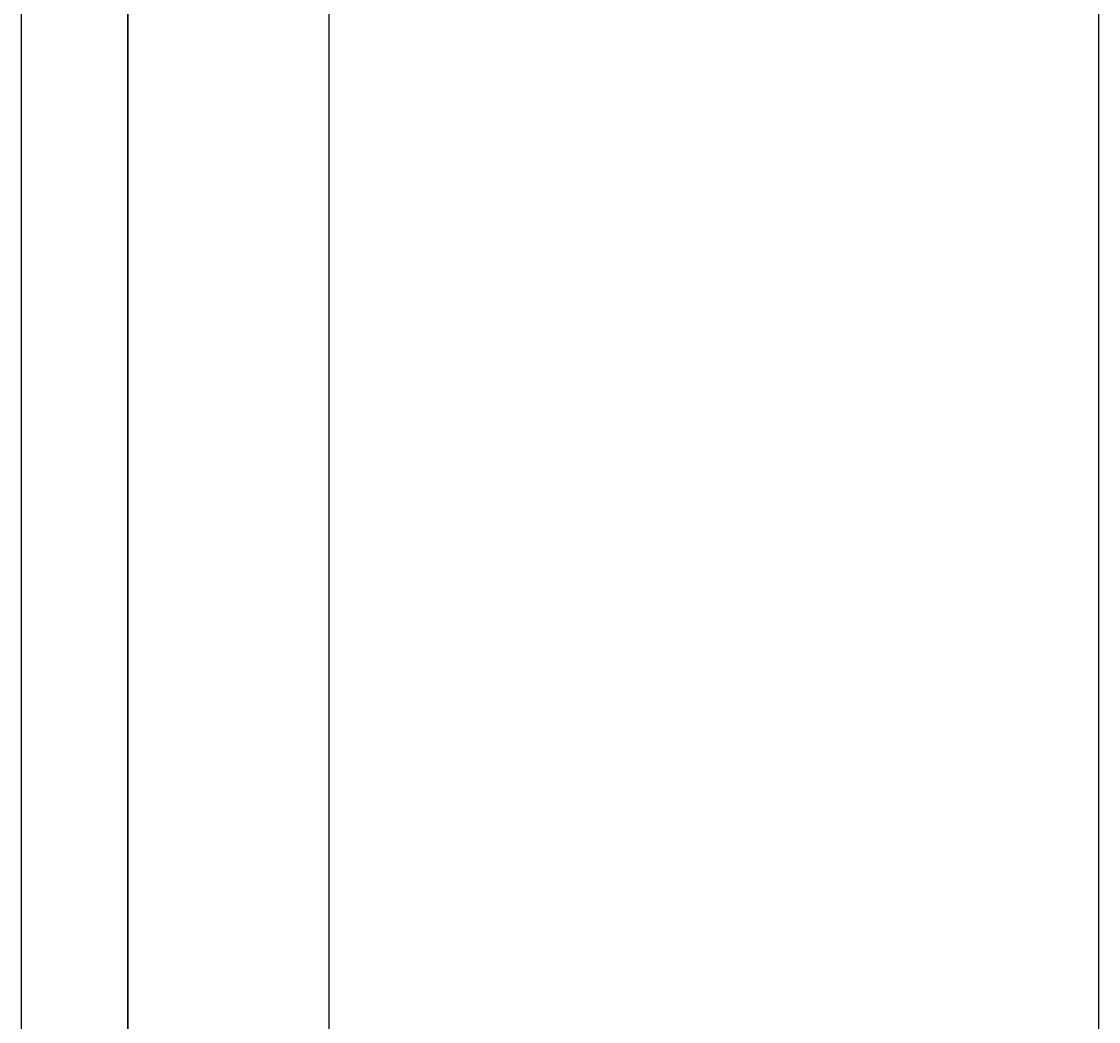
# Model space of a CAD drawing. Units: inches. Extents: x 2812 to 3051, y 1398 to 1659.
# Tile 25 of 65: x 2880 to 2911, y 1500 to 1528. Entities that reach past the tile are written whole.
import ezdxf

# ---------------------------------------------------------------- set-up
doc = ezdxf.new("R2010")
doc.units = ezdxf.units.IN
doc.layers.add('A-ANNO-DIMS', color=2, linetype='Continuous', lineweight=18)
doc.styles.get("Standard").update_dxf_attribs({"font": 'arial.ttf'})
doc.dimstyles.get("Standard").update_dxf_attribs({"dimtxt": 0.18, "dimasz": 0.18, "dimexe": 0.18, "dimexo": 0.0625, "dimgap": 0.09, "dimtad": 0, "dimtih": 1, "dimtoh": 1, "dimdec": 4, "dimzin": 0, "dimdsep": 46, "dimtxsty": 'Standard', "dimcen": 0.09, "dimadec": 0, "dimazin": 0, "dimtfac": 1, "dimtdec": 4, "dimtofl": 0, "dimtmove": 0, "dimatfit": 3, "dimfxl": 1, "dimtolj": 1, "dimtzin": 0, "dimarcsym": 0})

# ---------------------------------------------------------------- blocks, each defined once
blk = doc.blocks.new('*D29')
at = {"layer": 'A-ANNO-DIMS', "color": 0, "lineweight": -2, "transparency": 16777216}
for p, q in [((2910.742, 1598.757), (2910.742, 1397.505)), ((2883.385, 1559.757), (2883.385, 1397.505)), ((2883.565, 1397.685), (2896.598, 1397.685)), ((2910.562, 1397.685), (2897.528, 1397.685))]:
    blk.add_line(p, q, dxfattribs=at)
at = {"layer": 'A-ANNO-DIMS', "color": 0, "transparency": 16777216}
for points in [[(2883.565, 1397.715), (2883.565, 1397.655), (2883.385, 1397.685)], [(2910.562, 1397.715), (2910.562, 1397.655), (2910.742, 1397.685)]]:
    blk.add_solid(points, dxfattribs=at)
at = {"layer": 'Defpoints', "color": 0, "transparency": 16777216}
for p in [(2910.742, 1598.82), (2883.385, 1559.82), (2910.742, 1397.685)]:
    blk.add_point(p, dxfattribs=at)
at = {"layer": 'A-ANNO-DIMS', "color": 0, "transparency": 16777216, "insert": (2897.063, 1397.685), "char_height": 0.18, "attachment_point": 5}
blk.add_mtext('\\A1;27.357', dxfattribs=at)
blk = doc.blocks.new('*D58')
at = {"layer": 'A-ANNO-DIMS', "color": 0, "lineweight": -2, "transparency": 16777216}
for p, q in [((2880.385, 1472.098), (2880.385, 1659.35)), ((2883.385, 1472.098), (2883.385, 1659.35)), ((2880.565, 1659.17), (2881.736, 1659.17)), ((2883.205, 1659.17), (2882.034, 1659.17))]:
    blk.add_line(p, q, dxfattribs=at)
at = {"layer": 'A-ANNO-DIMS', "color": 0, "transparency": 16777216}
for points in [[(2880.565, 1659.2), (2880.565, 1659.14), (2880.385, 1659.17)], [(2883.205, 1659.2), (2883.205, 1659.14), (2883.385, 1659.17)]]:
    blk.add_solid(points, dxfattribs=at)
at = {"layer": 'Defpoints', "color": 0, "transparency": 16777216}
for p in [(2883.385, 1659.17), (2880.385, 1472.035), (2883.385, 1472.035)]:
    blk.add_point(p, dxfattribs=at)
at = {"layer": 'A-ANNO-DIMS', "color": 0, "transparency": 16777216, "insert": (2881.885, 1659.17), "char_height": 0.18, "attachment_point": 5}
blk.add_mtext('\\A1;3', dxfattribs=at)
blk = doc.blocks.new('*D59')
at = {"layer": 'A-ANNO-DIMS', "color": 0, "lineweight": -2, "transparency": 16777216}
for p, q in [((2883.385, 1452.098), (2883.385, 1659.35)), ((2889.058, 1467.465), (2889.058, 1659.35)), ((2883.565, 1659.17), (2885.828, 1659.17)), ((2888.878, 1659.17), (2886.615, 1659.17))]:
    blk.add_line(p, q, dxfattribs=at)
at = {"layer": 'A-ANNO-DIMS', "color": 0, "transparency": 16777216}
for points in [[(2883.565, 1659.2), (2883.565, 1659.14), (2883.385, 1659.17)], [(2888.878, 1659.2), (2888.878, 1659.14), (2889.058, 1659.17)]]:
    blk.add_solid(points, dxfattribs=at)
at = {"layer": 'Defpoints', "color": 0, "transparency": 16777216}
for p in [(2889.058, 1659.17), (2889.058, 1467.402), (2883.385, 1452.035)]:
    blk.add_point(p, dxfattribs=at)
at = {"layer": 'A-ANNO-DIMS', "color": 0, "transparency": 16777216, "insert": (2886.221, 1659.17), "char_height": 0.18, "attachment_point": 5}
blk.add_mtext('\\A1;5.673', dxfattribs=at)

msp = doc.modelspace()

# ---------------------------------------------------------------- dimensions: what is measured, and where the dimension line sits
at = {"layer": 'A-ANNO-DIMS'}
for base, p1, p2, override, picture, middle in [((2883.3849, 1659.17), (2880.3849, 1472.0354), (2883.3849, 1472.0354), {"dimdec": 0, "dimlfac": 1, "dimrnd": 0, "dimzin": 0, "dimdsep": 46, "dimlunit": 2}, '*D58', (2881.8849, 1659.17)), ((2889.0577, 1659.17), (2883.3849, 1452.0354), (2889.0577, 1467.4024), {"dimdec": 3, "dimlfac": 1, "dimrnd": 0, "dimzin": 0, "dimdsep": 46, "dimlunit": 2}, '*D59', (2886.2213, 1659.17)), ((2910.7415, 1397.6854), (2883.3849, 1559.82), (2910.7415, 1598.82), {"dimdec": 3, "dimlfac": 1, "dimrnd": 0, "dimzin": 0, "dimdsep": 46, "dimlunit": 2}, '*D29', (2897.0632, 1397.6854))]:
    dim = msp.add_linear_dim(base=base, p1=p1, p2=p2, dimstyle='Standard', override=override, dxfattribs=at)
    dim.commit()
    dim.dimension.update_dxf_attribs({"geometry": picture, "text_midpoint": middle})

doc.saveas('drawing.dxf')
